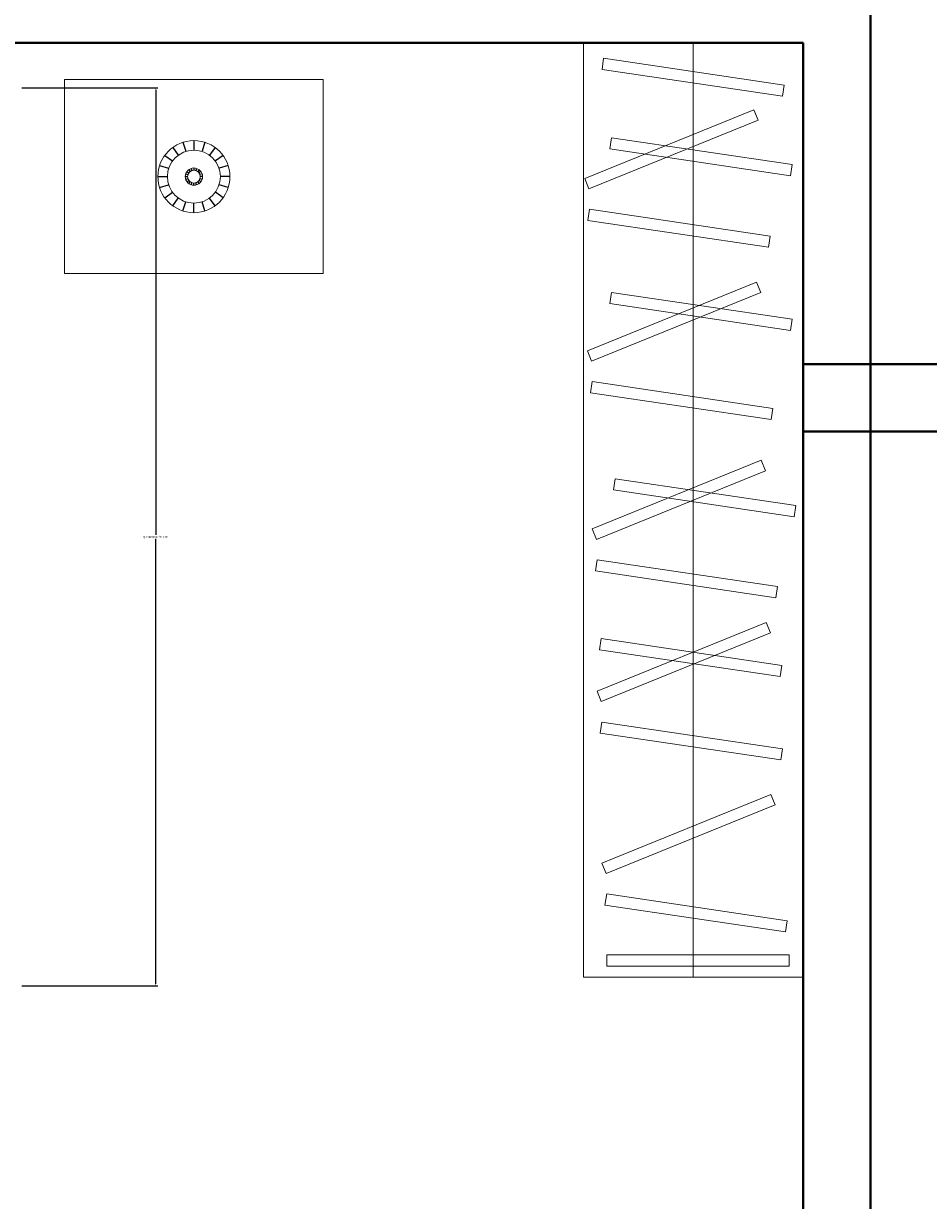
# Model space of a CAD drawing. Units: inches. Extents: x -46 to 1145, y -527 to 760.
# Tile 43 of 57: x 114 to 195, y 547 to 652. Entities that reach past the tile are written whole.
import ezdxf

# ---------------------------------------------------------------- set-up
doc = ezdxf.new("R2010")
doc.units = ezdxf.units.IN
doc.header["$MEASUREMENT"] = 0
for name, color, linetype, lineweight in [('A-ANNO-DIMS', 2, 'Continuous', 18), ('A-FLOR-CASE', 32, 'Continuous', 18), ('A-FURN', 2, 'Continuous', 13), ('WALLS', 4, 'Continuous', 40)]:
    doc.layers.add(name, color=color, linetype=linetype, lineweight=lineweight)
doc.layers.add('FURNTIURE', color=2, linetype='Continuous')
doc.styles.get("Standard").update_dxf_attribs({"font": 'arial.ttf'})
doc.dimstyles.get("Standard").update_dxf_attribs({"dimtxt": 0.18, "dimasz": 0.18, "dimexe": 0.18, "dimexo": 0.0625, "dimgap": 0.09, "dimtad": 0, "dimtih": 1, "dimtoh": 1, "dimdec": 0, "dimzin": 0, "dimdsep": 46, "dimlunit": 3, "dimtxsty": 'Standard', "dimcen": 0.09, "dimadec": 0, "dimazin": 0, "dimtfac": 1, "dimtdec": 0, "dimtofl": 0, "dimtmove": 0, "dimatfit": 3, "dimfxl": 1, "dimtolj": 1, "dimtzin": 0, "dimarcsym": 0})

# ---------------------------------------------------------------- blocks, each defined once
blk = doc.blocks.new('*U89')
at = {"layer": 'FURNTIURE'}
blk.add_line((0, 0.42), (0, -0.42), dxfattribs=at)
blk = doc.blocks.new('*U90')
at = {"layer": 'FURNTIURE', "transparency": 16777216}
for p, rotation in [((590.89, 507.4), 17.99999999999997), ((592.61, 507.4), 341.9999999999999), ((589.5, 506.39), 54), ((590.11, 507), 36), ((593.39, 507), 324), ((594.01, 506.39), 306), ((589.1, 505.61), 72), ((594.4, 505.61), 288), ((588.97, 504.75), 90), ((594.54, 504.75), 270), ((589.1, 503.89), 108), ((589.5, 503.11), 126), ((594.01, 503.11), 234), ((594.4, 503.89), 252), ((590.11, 502.49), 144), ((590.89, 502.1), 162), ((591.75, 501.96), 180), ((592.61, 502.1), 197.9999999999999), ((593.39, 502.49), 216)]:
    blk.add_blockref('*U89', p, dxfattribs=dict(at, rotation=rotation))
blk.add_blockref('*U89', (591.75, 507.53), dxfattribs=at)
blk = doc.blocks.new('*U87')
at = {"layer": 'FURNTIURE'}
blk.add_line((0, 0.1), (0, -0.1), dxfattribs=at)
blk = doc.blocks.new('*U88')
at = {"layer": 'FURNTIURE', "transparency": 16777216}
for p, rotation in [((141.51, 121.58), 35.99999999999999), ((141.7, 121.67), 17.99999999999998), ((142.11, 121.67), 342), ((142.3, 121.58), 324), ((141.23, 121.04), 90), ((141.27, 121.25), 72), ((141.27, 120.83), 108), ((141.36, 121.43), 54), ((141.36, 120.65), 126), ((142.44, 121.43), 306), ((142.44, 120.65), 234), ((142.54, 121.25), 288), ((142.54, 120.83), 252), ((142.57, 121.04), 270), ((141.51, 120.5), 144), ((141.7, 120.4), 162), ((141.9, 120.37), 180), ((142.11, 120.4), 198), ((142.3, 120.5), 216)]:
    blk.add_blockref('*U87', p, dxfattribs=dict(at, rotation=rotation))
blk.add_blockref('*U87', (141.9, 121.71), dxfattribs=at)
blk = doc.blocks.new('NIGHTSTAND')
blk.add_lwpolyline([(23.06, 0), (0, 0), (0, 17.28), (23.06, 17.28)], close=True)
for radius in [3.21, 2.36, 0.77, 0.567]:
    blk.add_circle((11.53, 8.64), radius)
for name, p in [('*U90', (-580.22, -496.1)), ('*U88', (-130.37, -112.4))]:
    blk.add_blockref(name, p)
blk = doc.blocks.new('WARDROBE')
blk.add_line((9.78, 0), (9.78, 83.25))
for points in [[(19.56, 0), (0, 0), (0, 83.25), (19.56, 83.25)], [(17.74, 78.49), (1.66, 80.88), (1.8, 81.87), (17.88, 79.48)], [(15.55, 76.35), (0.49, 70.23), (0.11, 71.16), (15.17, 77.28)], [(18.43, 71.4), (2.35, 73.79), (2.5, 74.78), (18.58, 72.39)], [(16.47, 65.03), (0.39, 67.42), (0.54, 68.41), (16.62, 66.02)], [(15.79, 61), (0.73, 54.88), (0.35, 55.81), (15.41, 61.93)], [(18.43, 57.62), (2.35, 60.01), (2.5, 61), (18.58, 58.61)], [(16.71, 49.68), (0.63, 52.07), (0.78, 53.06), (16.86, 50.67)], [(16.22, 45.12), (1.16, 39), (0.78, 39.93), (15.84, 46.05)], [(18.77, 41.02), (2.69, 43.41), (2.84, 44.4), (18.92, 42.01)], [(17.14, 33.8), (1.06, 36.19), (1.21, 37.19), (17.29, 34.8)], [(16.65, 30.67), (1.59, 24.55), (1.21, 25.48), (16.27, 31.6)], [(17.52, 26.78), (1.44, 29.17), (1.59, 30.16), (17.67, 27.77)], [(17.57, 19.35), (1.49, 21.74), (1.64, 22.73), (17.72, 20.34)], [(17.08, 15.35), (2.02, 9.23), (1.64, 10.16), (16.7, 16.28)], [(18, 4.03), (1.92, 6.42), (2.07, 7.41), (18.15, 5.03)], [(18.32, 0.98), (2.07, 0.98), (2.07, 1.98), (18.32, 1.98)]]:
    blk.add_lwpolyline(points, close=True)
blk = doc.blocks.new('*D652')
at = {"layer": 'A-ANNO-DIMS', "color": 0, "lineweight": -2, "transparency": 16777216}
for p, q in [((113.97, 646.5), (126.09, 646.5)), ((125.91, 646.32), (125.91, 606.69)), ((125.91, 566.68), (125.91, 606.31)), ((113.97, 566.5), (126.09, 566.5))]:
    blk.add_line(p, q, dxfattribs=at)
at = {"layer": 'A-ANNO-DIMS', "color": 0, "transparency": 16777216}
for points in [[(125.88, 646.32), (125.94, 646.32), (125.91, 646.5)], [(125.88, 566.68), (125.94, 566.68), (125.91, 566.5)]]:
    blk.add_solid(points, dxfattribs=at)
at = {"layer": 'Defpoints', "color": 0, "transparency": 16777216}
for p in [(113.91, 646.5), (125.91, 646.5), (113.91, 566.5)]:
    blk.add_point(p, dxfattribs=at)
at = {"layer": 'A-ANNO-DIMS', "color": 0, "transparency": 16777216, "insert": (125.91, 606.5), "char_height": 0.18, "attachment_point": 5}
blk.add_mtext('\\A1;QUEEN BED 80 TYP.', dxfattribs=at)
blk = doc.blocks.new('*D685')
at = {"layer": 'A-ANNO-DIMS', "color": 0, "lineweight": -2, "transparency": 16777216}
for p, q in [((183.5, 700.89), (-46.22, 700.89)), ((-46.04, 700.71), (-46.04, 116.39)), ((-46.04, -468.3), (-46.04, 116.02)), ((12.5, -468.48), (-46.22, -468.48))]:
    blk.add_line(p, q, dxfattribs=at)
at = {"layer": 'A-ANNO-DIMS', "color": 0, "transparency": 16777216}
for points in [[(-46.07, 700.71), (-46.01, 700.71), (-46.04, 700.89)], [(-46.07, -468.3), (-46.01, -468.3), (-46.04, -468.48)]]:
    blk.add_solid(points, dxfattribs=at)
at = {"layer": 'Defpoints', "color": 0, "transparency": 16777216}
for p in [(-46.04, 700.89), (183.56, 700.89), (12.56, -468.48)]:
    blk.add_point(p, dxfattribs=at)
at = {"layer": 'A-ANNO-DIMS', "color": 0, "transparency": 16777216, "insert": (-46.04, 116.2), "char_height": 0.18, "attachment_point": 5}
blk.add_mtext('\\A1;1169.4', dxfattribs=at)

msp = doc.modelspace()

# ---------------------------------------------------------------- linework, layer by layer
at = {"layer": 'WALLS'}
for p, q in [((189.5637, 659.5176), (189.5637, 500.5176)), ((183.5637, 650.5176), (21.5637, 650.5176)), ((183.5637, 650.5176), (183.5637, 506.5176)), ((183.5637, 621.8886), (333.5637, 621.8886)), ((183.5637, 615.8886), (333.5637, 615.8886))]:
    msp.add_line(p, q, dxfattribs=at)

# ---------------------------------------------------------------- block references
at = {"layer": 'A-FLOR-CASE'}
msp.add_blockref('WARDROBE', (164.004, 567.272), dxfattribs=at)
at = {"layer": 'A-FURN'}
msp.add_blockref('NIGHTSTAND', (117.7733, 629.954), dxfattribs=at)

# ---------------------------------------------------------------- dimensions: what is measured, and where the dimension line sits
at = {"layer": 'A-ANNO-DIMS'}
dim = msp.add_linear_dim(base=(-46.0363, 700.8886), p1=(12.5637, -468.4824), p2=(183.5637, 700.8886), angle=90, dimstyle='Standard', override={"dimdec": 1, "dimlfac": 1, "dimrnd": 0, "dimzin": 0, "dimdsep": 46, "dimlunit": 2}, dxfattribs=at)
dim.commit()
dim.dimension.update_dxf_attribs({"geometry": '*D685', "text_midpoint": (-46.0363, 116.2031)})
dim = msp.add_linear_dim(base=(125.9098, 646.5029), p1=(113.9098, 566.5028), p2=(113.9098, 646.5029), angle=90, text='QUEEN BED <> TYP.', dimstyle='Standard', override={"dimdec": 0, "dimlfac": 1, "dimrnd": 0, "dimzin": 0, "dimdsep": 46, "dimlunit": 2}, dxfattribs=at)
dim.commit()
dim.dimension.update_dxf_attribs({"geometry": '*D652', "text_midpoint": (125.9098, 606.5028)})

doc.saveas('drawing.dxf')
